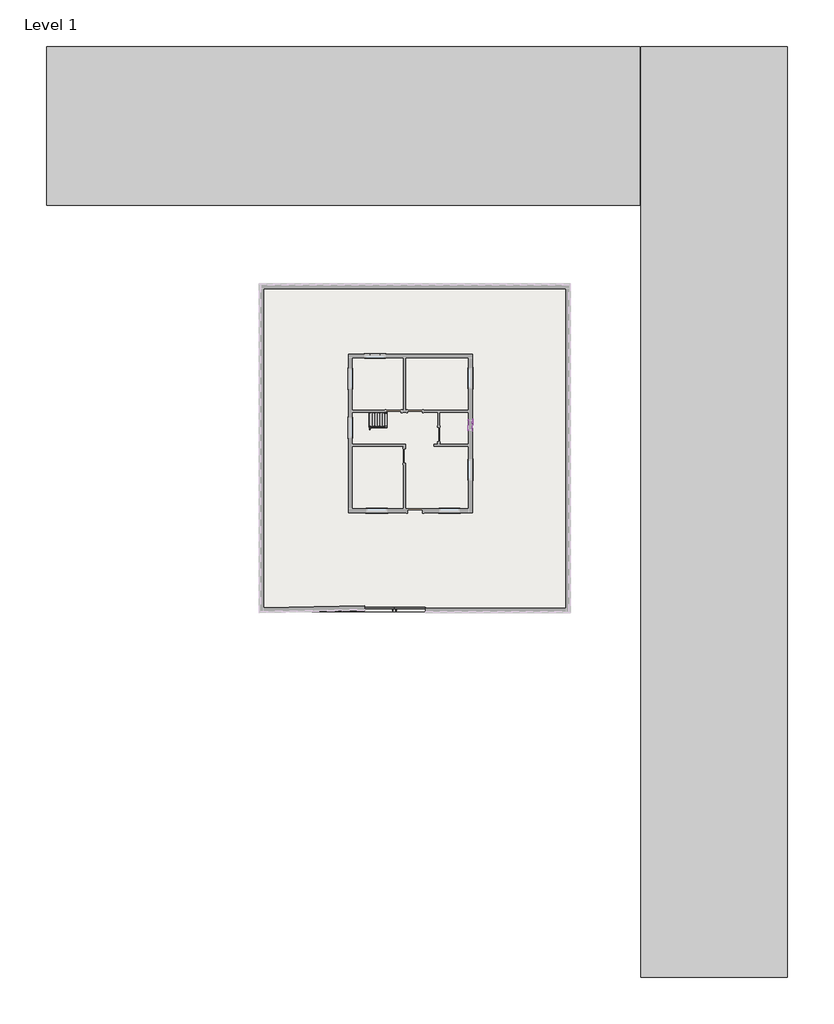
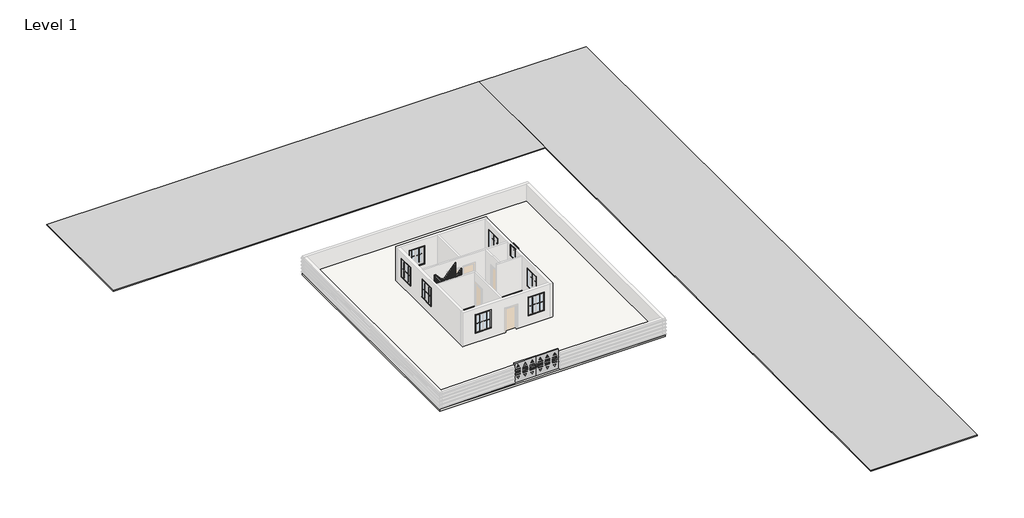
# One storey, part 2 of 2: 35 proxies, 3 members, 2 railings, 1 slab, 1 stair flight.
"""IFC4 building model written with IfcOpenShell, lengths in millimetres."""

from ifc_helpers import new_model, si_unit, frame, origin, place, context, project, spatial, polyline, outline, extrude, faceted_brep, transform, mapped, element, save
from components import generic_models_afecbd1f, generic_models_1_generic_models_1_344866f9, generic_models_2_generic_models_2_ab047e66, muntin_pattern_2x2_muntin_pattern_2x2_6dad3731, muntin_pattern_2x2_muntin_pattern_2x2_a30a3345, muntin_pattern_2x2_muntin_pattern_2x2_53152e2c, muntin_pattern_2x2_muntin_pattern_2x2_e8f3e573, trim_window_exterior_flat_with_sill_92b9b949, trim_window_exterior_flat_with_sill_a665a915, trim_window_interior_flat_picture_frame_3bb882cf, trim_window_interior_flat_picture_frame_d485c387, stair_flight_41b76c56

model = new_model("IFC4")

# Units and contexts
model_context = context("Model", 3, world=origin())
ifc_project = project(units=[si_unit("LENGTHUNIT", "METRE", prefix="MILLI")], contexts=[model_context])

# Site, building, storey
site = spatial("IfcSite", under=ifc_project)
building = spatial("IfcBuilding", under=site)
storey = spatial("IfcBuildingStorey", under=building, Name="Level 1", Elevation=0.0)

# Proxies
placement = place(None, origin())
generic_models_shape = generic_models_afecbd1f(model_context)
element("IfcBuildingElementProxy", 1, Name="Generic Models", at=placement, inside=storey, context=model_context, shape_type="MappedRepresentation", body=[
    mapped(generic_models_shape, transform((3790.95, -1079.5, 0.0), x_axis=(1.0, 0.0, 0.0), y_axis=(0.0, 1.0, 0.0), z_axis=(0.0, 0.0, 1.0))),
])
generic_models_1_generic_models_1_shape = generic_models_1_generic_models_1_344866f9(model_context)
element("IfcBuildingElementProxy", 2, Name="Generic Models 1 : Generic Models 1", ObjectType="Generic Models 1 : Generic Models 1", at=placement, inside=storey, context=model_context, shape_type="MappedRepresentation", body=[
    mapped(generic_models_1_generic_models_1_shape, transform((0.0, 0.0, 0.0), x_axis=(1.0, 0.0, 0.0), y_axis=(0.0, 1.0, 0.0), z_axis=(0.0, 0.0, 1.0))),
])
generic_models_2_generic_models_2_shape = generic_models_2_generic_models_2_ab047e66(model_context)
element("IfcBuildingElementProxy", 3, Name="Generic Models 2 : Generic Models 2", ObjectType="Generic Models 2 : Generic Models 2", at=placement, inside=storey, context=model_context, shape_type="MappedRepresentation", body=[
    mapped(generic_models_2_generic_models_2_shape, transform((0.0, 0.0, 0.0), x_axis=(1.0, 0.0, 0.0), y_axis=(0.0, 1.0, 0.0), z_axis=(0.0, 0.0, 1.0))),
])
muntin_pattern_2x2_muntin_pattern_2x2_shape = muntin_pattern_2x2_muntin_pattern_2x2_6dad3731(model_context)
element("IfcBuildingElementProxy", 4, Name="Muntin Pattern_2x2 : Muntin Pattern_2x2", ObjectType="Muntin Pattern_2x2 : Muntin Pattern_2x2", at=placement, inside=storey, context=model_context, shape_type="MappedRepresentation", body=[
    mapped(muntin_pattern_2x2_muntin_pattern_2x2_shape, transform((2601.9125, 14468.475, 984.25), x_axis=(1.0, 0.0, 0.0), y_axis=(0.0, 1.0, 0.0), z_axis=(0.0, 0.0, 1.0))),
])
element("IfcBuildingElementProxy", 5, Name="Muntin Pattern_2x2 : Muntin Pattern_2x2", ObjectType="Muntin Pattern_2x2 : Muntin Pattern_2x2", at=placement, inside=storey, context=model_context, shape_type="MappedRepresentation", body=[
    mapped(muntin_pattern_2x2_muntin_pattern_2x2_shape, transform((8880.475, 13295.3125, 984.25), x_axis=(0.0, -1.0, 0.0), y_axis=(1.0, 0.0, 0.0), z_axis=(0.0, 0.0, 1.0))),
])
element("IfcBuildingElementProxy", 6, Name="Muntin Pattern_2x2 : Muntin Pattern_2x2", ObjectType="Muntin Pattern_2x2 : Muntin Pattern_2x2", at=placement, inside=storey, context=model_context, shape_type="MappedRepresentation", body=[
    mapped(muntin_pattern_2x2_muntin_pattern_2x2_shape, transform((8880.475, 7662.8625, 984.25), x_axis=(0.0, -1.0, 0.0), y_axis=(1.0, 0.0, 0.0), z_axis=(0.0, 0.0, 1.0))),
])
element("IfcBuildingElementProxy", 7, Name="Muntin Pattern_2x2 : Muntin Pattern_2x2", ObjectType="Muntin Pattern_2x2 : Muntin Pattern_2x2", at=placement, inside=storey, context=model_context, shape_type="MappedRepresentation", body=[
    mapped(muntin_pattern_2x2_muntin_pattern_2x2_shape, transform((7785.1, 4733.925, 984.25), x_axis=(-1.0, 0.0, 0.0), y_axis=(0.0, -1.0, 0.0), z_axis=(0.0, 0.0, 1.0))),
])
element("IfcBuildingElementProxy", 8, Name="Muntin Pattern_2x2 : Muntin Pattern_2x2", ObjectType="Muntin Pattern_2x2 : Muntin Pattern_2x2", at=placement, inside=storey, context=model_context, shape_type="MappedRepresentation", body=[
    mapped(muntin_pattern_2x2_muntin_pattern_2x2_shape, transform((3313.1125, 4733.925, 984.25), x_axis=(-1.0, 0.0, 0.0), y_axis=(0.0, -1.0, 0.0), z_axis=(0.0, 0.0, 1.0))),
])
element("IfcBuildingElementProxy", 9, Name="Muntin Pattern_2x2 : Muntin Pattern_2x2", ObjectType="Muntin Pattern_2x2 : Muntin Pattern_2x2", at=placement, inside=storey, context=model_context, shape_type="MappedRepresentation", body=[
    mapped(muntin_pattern_2x2_muntin_pattern_2x2_shape, transform((1279.525, 9647.2375, 984.25), x_axis=(0.0, 1.0, 0.0), y_axis=(-1.0, 0.0, 0.0), z_axis=(0.0, 0.0, 1.0))),
])
element("IfcBuildingElementProxy", 10, Name="Muntin Pattern_2x2 : Muntin Pattern_2x2", ObjectType="Muntin Pattern_2x2 : Muntin Pattern_2x2", at=placement, inside=storey, context=model_context, shape_type="MappedRepresentation", body=[
    mapped(muntin_pattern_2x2_muntin_pattern_2x2_shape, transform((1279.525, 12657.1375, 984.25), x_axis=(0.0, 1.0, 0.0), y_axis=(-1.0, 0.0, 0.0), z_axis=(0.0, 0.0, 1.0))),
])
muntin_pattern_2x2_muntin_pattern_2x2_2_shape = muntin_pattern_2x2_muntin_pattern_2x2_a30a3345(model_context)
element("IfcBuildingElementProxy", 11, Name="Muntin Pattern_2x2 : Muntin Pattern_2x2", ObjectType="Muntin Pattern_2x2 : Muntin Pattern_2x2", at=placement, inside=storey, context=model_context, shape_type="MappedRepresentation", body=[
    mapped(muntin_pattern_2x2_muntin_pattern_2x2_2_shape, transform((3208.3375, 14468.475, 984.25), x_axis=(-1.0, 0.0, 0.0), y_axis=(0.0, -1.0, 0.0), z_axis=(0.0, 0.0, 1.0))),
])
element("IfcBuildingElementProxy", 12, Name="Muntin Pattern_2x2 : Muntin Pattern_2x2", ObjectType="Muntin Pattern_2x2 : Muntin Pattern_2x2", at=placement, inside=storey, context=model_context, shape_type="MappedRepresentation", body=[
    mapped(muntin_pattern_2x2_muntin_pattern_2x2_2_shape, transform((8880.475, 12688.8875, 984.25), x_axis=(0.0, 1.0, 0.0), y_axis=(-1.0, 0.0, 0.0), z_axis=(0.0, 0.0, 1.0))),
])
element("IfcBuildingElementProxy", 13, Name="Muntin Pattern_2x2 : Muntin Pattern_2x2", ObjectType="Muntin Pattern_2x2 : Muntin Pattern_2x2", at=placement, inside=storey, context=model_context, shape_type="MappedRepresentation", body=[
    mapped(muntin_pattern_2x2_muntin_pattern_2x2_2_shape, transform((8880.475, 7056.4375, 984.25), x_axis=(0.0, 1.0, 0.0), y_axis=(-1.0, 0.0, 0.0), z_axis=(0.0, 0.0, 1.0))),
])
element("IfcBuildingElementProxy", 14, Name="Muntin Pattern_2x2 : Muntin Pattern_2x2", ObjectType="Muntin Pattern_2x2 : Muntin Pattern_2x2", at=placement, inside=storey, context=model_context, shape_type="MappedRepresentation", body=[
    mapped(muntin_pattern_2x2_muntin_pattern_2x2_2_shape, transform((7178.675, 4733.925, 984.25), x_axis=(1.0, 0.0, 0.0), y_axis=(0.0, 1.0, 0.0), z_axis=(0.0, 0.0, 1.0))),
])
element("IfcBuildingElementProxy", 15, Name="Muntin Pattern_2x2 : Muntin Pattern_2x2", ObjectType="Muntin Pattern_2x2 : Muntin Pattern_2x2", at=placement, inside=storey, context=model_context, shape_type="MappedRepresentation", body=[
    mapped(muntin_pattern_2x2_muntin_pattern_2x2_2_shape, transform((2706.6875, 4733.925, 984.25), x_axis=(1.0, 0.0, 0.0), y_axis=(0.0, 1.0, 0.0), z_axis=(0.0, 0.0, 1.0))),
])
element("IfcBuildingElementProxy", 16, Name="Muntin Pattern_2x2 : Muntin Pattern_2x2", ObjectType="Muntin Pattern_2x2 : Muntin Pattern_2x2", at=placement, inside=storey, context=model_context, shape_type="MappedRepresentation", body=[
    mapped(muntin_pattern_2x2_muntin_pattern_2x2_2_shape, transform((1279.525, 10253.6625, 984.25), x_axis=(0.0, -1.0, 0.0), y_axis=(1.0, 0.0, 0.0), z_axis=(0.0, 0.0, 1.0))),
])
element("IfcBuildingElementProxy", 17, Name="Muntin Pattern_2x2 : Muntin Pattern_2x2", ObjectType="Muntin Pattern_2x2 : Muntin Pattern_2x2", at=placement, inside=storey, context=model_context, shape_type="MappedRepresentation", body=[
    mapped(muntin_pattern_2x2_muntin_pattern_2x2_2_shape, transform((1279.525, 13263.5625, 984.25), x_axis=(0.0, -1.0, 0.0), y_axis=(1.0, 0.0, 0.0), z_axis=(0.0, 0.0, 1.0))),
])
muntin_pattern_2x2_muntin_pattern_2x2_3_shape = muntin_pattern_2x2_muntin_pattern_2x2_53152e2c(model_context)
element("IfcBuildingElementProxy", 18, Name="Muntin Pattern_2x2 : Muntin Pattern_2x2", ObjectType="Muntin Pattern_2x2 : Muntin Pattern_2x2", at=placement, inside=storey, context=model_context, shape_type="MappedRepresentation", body=[
    mapped(muntin_pattern_2x2_muntin_pattern_2x2_3_shape, transform((8880.475, 10266.3625, 2203.45), x_axis=(0.0, -1.0, 0.0), y_axis=(1.0, 0.0, 0.0), z_axis=(0.0, 0.0, 1.0))),
])
muntin_pattern_2x2_muntin_pattern_2x2_4_shape = muntin_pattern_2x2_muntin_pattern_2x2_e8f3e573(model_context)
element("IfcBuildingElementProxy", 19, Name="Muntin Pattern_2x2 : Muntin Pattern_2x2", ObjectType="Muntin Pattern_2x2 : Muntin Pattern_2x2", at=placement, inside=storey, context=model_context, shape_type="MappedRepresentation", body=[
    mapped(muntin_pattern_2x2_muntin_pattern_2x2_4_shape, transform((8880.475, 9964.7375, 2203.45), x_axis=(0.0, 1.0, 0.0), y_axis=(-1.0, 0.0, 0.0), z_axis=(0.0, 0.0, 1.0))),
])
trim_window_exterior_flat_with_sill_shape = trim_window_exterior_flat_with_sill_92b9b949(model_context)
element("IfcBuildingElementProxy", 20, Name="Trim-Window-Exterior-Flat : with Sill", ObjectType="Trim-Window-Exterior-Flat : with Sill", at=placement, inside=storey, context=model_context, shape_type="MappedRepresentation", body=[
    mapped(trim_window_exterior_flat_with_sill_shape, transform((2905.125, 14478.0, 2438.4), x_axis=(-1.0, 0.0, 0.0), y_axis=(0.0, 0.0, 1.0), z_axis=(0.0, 1.0, 0.0))),
])
element("IfcBuildingElementProxy", 21, Name="Trim-Window-Exterior-Flat : with Sill", ObjectType="Trim-Window-Exterior-Flat : with Sill", at=placement, inside=storey, context=model_context, shape_type="MappedRepresentation", body=[
    mapped(trim_window_exterior_flat_with_sill_shape, transform((8890.0, 12992.1, 2438.4), x_axis=(0.0, 1.0, 0.0), y_axis=(0.0, 0.0, 1.0), z_axis=(1.0, 0.0, 0.0))),
])
element("IfcBuildingElementProxy", 22, Name="Trim-Window-Exterior-Flat : with Sill", ObjectType="Trim-Window-Exterior-Flat : with Sill", at=placement, inside=storey, context=model_context, shape_type="MappedRepresentation", body=[
    mapped(trim_window_exterior_flat_with_sill_shape, transform((8890.0, 7359.65, 2438.4), x_axis=(0.0, 1.0, 0.0), y_axis=(0.0, 0.0, 1.0), z_axis=(1.0, 0.0, 0.0))),
])
element("IfcBuildingElementProxy", 23, Name="Trim-Window-Exterior-Flat : with Sill", ObjectType="Trim-Window-Exterior-Flat : with Sill", at=placement, inside=storey, context=model_context, shape_type="MappedRepresentation", body=[
    mapped(trim_window_exterior_flat_with_sill_shape, transform((7481.8875, 4724.4, 2438.4), x_axis=(1.0, 0.0, 0.0), y_axis=(0.0, 0.0, 1.0), z_axis=(0.0, -1.0, 0.0))),
])
element("IfcBuildingElementProxy", 24, Name="Trim-Window-Exterior-Flat : with Sill", ObjectType="Trim-Window-Exterior-Flat : with Sill", at=placement, inside=storey, context=model_context, shape_type="MappedRepresentation", body=[
    mapped(trim_window_exterior_flat_with_sill_shape, transform((3009.9, 4724.4, 2438.4), x_axis=(1.0, 0.0, 0.0), y_axis=(0.0, 0.0, 1.0), z_axis=(0.0, -1.0, 0.0))),
])
element("IfcBuildingElementProxy", 25, Name="Trim-Window-Exterior-Flat : with Sill", ObjectType="Trim-Window-Exterior-Flat : with Sill", at=placement, inside=storey, context=model_context, shape_type="MappedRepresentation", body=[
    mapped(trim_window_exterior_flat_with_sill_shape, transform((1270.0, 9950.45, 2438.4), x_axis=(0.0, -1.0, 0.0), y_axis=(0.0, 0.0, 1.0), z_axis=(-1.0, 0.0, 0.0))),
])
element("IfcBuildingElementProxy", 26, Name="Trim-Window-Exterior-Flat : with Sill", ObjectType="Trim-Window-Exterior-Flat : with Sill", at=placement, inside=storey, context=model_context, shape_type="MappedRepresentation", body=[
    mapped(trim_window_exterior_flat_with_sill_shape, transform((1270.0, 12960.35, 2438.4), x_axis=(0.0, -1.0, 0.0), y_axis=(0.0, 0.0, 1.0), z_axis=(-1.0, 0.0, 0.0))),
])
trim_window_exterior_flat_with_sill_2_shape = trim_window_exterior_flat_with_sill_a665a915(model_context)
element("IfcBuildingElementProxy", 27, Name="Trim-Window-Exterior-Flat : with Sill", ObjectType="Trim-Window-Exterior-Flat : with Sill", at=placement, inside=storey, context=model_context, shape_type="MappedRepresentation", body=[
    mapped(trim_window_exterior_flat_with_sill_2_shape, transform((8890.0, 10115.55, 3048.0), x_axis=(0.0, 1.0, 0.0), y_axis=(0.0, 0.0, 1.0), z_axis=(1.0, 0.0, 0.0))),
])
trim_window_interior_flat_picture_frame_shape = trim_window_interior_flat_picture_frame_3bb882cf(model_context)
element("IfcBuildingElementProxy", 28, Name="Trim-Window-Interior-Flat : Picture Frame", ObjectType="Trim-Window-Interior-Flat : Picture Frame", at=placement, inside=storey, context=model_context, shape_type="MappedRepresentation", body=[
    mapped(trim_window_interior_flat_picture_frame_shape, transform((2905.125, 14249.4, 2438.4), x_axis=(1.0, 0.0, 0.0), y_axis=(0.0, 0.0, 1.0), z_axis=(0.0, -1.0, 0.0))),
])
element("IfcBuildingElementProxy", 29, Name="Trim-Window-Interior-Flat : Picture Frame", ObjectType="Trim-Window-Interior-Flat : Picture Frame", at=placement, inside=storey, context=model_context, shape_type="MappedRepresentation", body=[
    mapped(trim_window_interior_flat_picture_frame_shape, transform((8661.4, 12992.1, 2438.4), x_axis=(0.0, -1.0, 0.0), y_axis=(0.0, 0.0, 1.0), z_axis=(-1.0, 0.0, 0.0))),
])
element("IfcBuildingElementProxy", 30, Name="Trim-Window-Interior-Flat : Picture Frame", ObjectType="Trim-Window-Interior-Flat : Picture Frame", at=placement, inside=storey, context=model_context, shape_type="MappedRepresentation", body=[
    mapped(trim_window_interior_flat_picture_frame_shape, transform((8661.4, 7359.65, 2438.4), x_axis=(0.0, -1.0, 0.0), y_axis=(0.0, 0.0, 1.0), z_axis=(-1.0, 0.0, 0.0))),
])
element("IfcBuildingElementProxy", 31, Name="Trim-Window-Interior-Flat : Picture Frame", ObjectType="Trim-Window-Interior-Flat : Picture Frame", at=placement, inside=storey, context=model_context, shape_type="MappedRepresentation", body=[
    mapped(trim_window_interior_flat_picture_frame_shape, transform((7481.8875, 4953.0, 2438.4), x_axis=(-1.0, 0.0, 0.0), y_axis=(0.0, 0.0, 1.0), z_axis=(0.0, 1.0, 0.0))),
])
element("IfcBuildingElementProxy", 32, Name="Trim-Window-Interior-Flat : Picture Frame", ObjectType="Trim-Window-Interior-Flat : Picture Frame", at=placement, inside=storey, context=model_context, shape_type="MappedRepresentation", body=[
    mapped(trim_window_interior_flat_picture_frame_shape, transform((3009.9, 4953.0, 2438.4), x_axis=(-1.0, 0.0, 0.0), y_axis=(0.0, 0.0, 1.0), z_axis=(0.0, 1.0, 0.0))),
])
element("IfcBuildingElementProxy", 33, Name="Trim-Window-Interior-Flat : Picture Frame", ObjectType="Trim-Window-Interior-Flat : Picture Frame", at=placement, inside=storey, context=model_context, shape_type="MappedRepresentation", body=[
    mapped(trim_window_interior_flat_picture_frame_shape, transform((1498.6, 9950.45, 2438.4), x_axis=(0.0, 1.0, 0.0), y_axis=(0.0, 0.0, 1.0), z_axis=(1.0, 0.0, 0.0))),
])
element("IfcBuildingElementProxy", 34, Name="Trim-Window-Interior-Flat : Picture Frame", ObjectType="Trim-Window-Interior-Flat : Picture Frame", at=placement, inside=storey, context=model_context, shape_type="MappedRepresentation", body=[
    mapped(trim_window_interior_flat_picture_frame_shape, transform((1498.6, 12960.35, 2438.4), x_axis=(0.0, 1.0, 0.0), y_axis=(0.0, 0.0, 1.0), z_axis=(1.0, 0.0, 0.0))),
])
trim_window_interior_flat_picture_frame_2_shape = trim_window_interior_flat_picture_frame_d485c387(model_context)
element("IfcBuildingElementProxy", 35, Name="Trim-Window-Interior-Flat : Picture Frame", ObjectType="Trim-Window-Interior-Flat : Picture Frame", at=placement, inside=storey, context=model_context, shape_type="MappedRepresentation", body=[
    mapped(trim_window_interior_flat_picture_frame_2_shape, transform((8661.4, 10115.55, 3048.0), x_axis=(0.0, -1.0, 0.0), y_axis=(0.0, 0.0, 1.0), z_axis=(-1.0, 0.0, 0.0))),
])

# Members
element("IfcMember", 36, ObjectType="Stringer - 2\" Width", at=placement, inside=storey, context=model_context, shape_type="SweptSolid", body=[
    extrude(outline(polyline([(0.0, 3632.2), (274.6288314, 3632.2), (1403.5177203, 2616.2), (947.8883192, 2616.2), (0.0, 3469.2994873), (0.0, 3632.2)])), frame((0.0, 9944.1, 0.0), z_axis=(0.0, 1.0, 0.0), x_axis=(0.0, 0.0, 1.0)), (0.0, 0.0, 1.0), 50.8),
])
element("IfcMember", 37, ObjectType="Stringer - 2\" Width", at=placement, inside=storey, context=model_context, shape_type="SweptSolid", body=[
    extrude(outline(polyline([(2565.4, 9994.9), (2616.2, 9994.9), (2616.2, 9893.3), (2565.4, 9893.3), (2565.4, 9994.9)])), frame((0.0, 0.0, 1126.0666667), z_axis=(0.0, 0.0, 1.0), x_axis=(1.0, 0.0, 0.0)), (0.0, 0.0, 1.0), 304.8),
])
element("IfcMember", 38, ObjectType="Stringer - 2\" Width", at=placement, inside=storey, context=model_context, shape_type="SweptSolid", body=[
    extrude(outline(polyline([(1629.2954981, 2565.4), (1173.666097, 2565.4), (2358.9994303, 3632.2), (2814.6288314, 3632.2), (1629.2954981, 2565.4)])), frame((0.0, 9842.5, 0.0), z_axis=(0.0, 1.0, 0.0), x_axis=(0.0, 0.0, 1.0)), (0.0, 0.0, 1.0), 50.8),
])

# Railings
element("IfcRailing", 39, ObjectType="Handrail - Rectangular", at=placement, inside=storey, context=model_context, shape_type="SolidModel", body=[
    faceted_brep([(3632.2, 10858.5, 1083.7333333), (3632.2, 10858.5, 1007.7950998), (3632.2, 10909.3, 1007.7950998), (3632.2, 10909.3, 1083.7333333), (2565.4, 10858.5, 2269.0666667), (2542.7755898, 10858.5, 2218.2666667), (2542.7755898, 10909.3, 2218.2666667), (2565.4, 10909.3, 2269.0666667), (2463.8, 10858.5, 2269.0666667), (2463.8, 10858.5, 2218.2666667), (2413.0, 10909.3, 2218.2666667), (2413.0, 10909.3, 2269.0666667), (2463.8, 9055.1, 2269.0666667), (2463.8, 9004.3, 2218.2666667), (2413.0, 9004.3, 2218.2666667), (2413.0, 9055.1, 2269.0666667), (2463.8, 9055.1, 2410.1777778), (2463.8, 9004.3, 2359.3777778), (2413.0, 9004.3, 2359.3777778), (2413.0, 9055.1, 2410.1777778), (2463.8, 8978.9, 2410.1777778), (2463.8, 8978.9, 2359.3777778), (2413.0, 8928.1, 2359.3777778), (2413.0, 8928.1, 2410.1777778), (2540.0, 8978.9, 2410.1777778), (2562.6244102, 8978.9, 2359.3777778), (2562.6244102, 8928.1, 2359.3777778), (2540.0, 8928.1, 2410.1777778), (3632.2, 8978.9, 3623.7333333), (3632.2, 8928.1, 3623.7333333), (3632.2, 8928.1, 3547.7950998), (3632.2, 8978.9, 3547.7950998)], [[[0, 1, 2, 3]], [[1, 0, 4, 5]], [[2, 1, 5, 6]], [[3, 2, 6, 7]], [[0, 3, 7, 4]], [[5, 4, 8, 9]], [[6, 5, 9, 10]], [[7, 6, 10, 11]], [[4, 7, 11, 8]], [[9, 8, 12, 13]], [[10, 9, 13, 14]], [[11, 10, 14, 15]], [[8, 11, 15, 12]], [[13, 12, 16, 17]], [[14, 13, 17, 18]], [[15, 14, 18, 19]], [[12, 15, 19, 16]], [[17, 16, 20, 21]], [[18, 17, 21, 22]], [[19, 18, 22, 23]], [[16, 19, 23, 20]], [[21, 20, 24, 25]], [[22, 21, 25, 26]], [[23, 22, 26, 27]], [[20, 23, 27, 24]], [[28, 29, 30, 31]], [[25, 24, 28, 31]], [[26, 25, 31, 30]], [[27, 26, 30, 29]], [[24, 27, 29, 28]]]),
    extrude(outline(polyline([(3473.7117665, 3565.525), (3452.5450998, 3546.475), (2540.0, 3546.475), (2540.0, 3565.525), (3473.7117665, 3565.525)])), frame((0.0, 8943.975, 0.0), z_axis=(0.0, 1.0, 0.0), x_axis=(0.0, 0.0, 1.0)), (0.0, 0.0, 1.0), 19.05),
    extrude(outline(polyline([(3360.8228776, 3463.925), (3339.6562109, 3444.875), (2370.6666667, 3444.875), (2370.6666667, 3463.925), (3360.8228776, 3463.925)])), frame((0.0, 8943.975, 0.0), z_axis=(0.0, 1.0, 0.0), x_axis=(0.0, 0.0, 1.0)), (0.0, 0.0, 1.0), 19.05),
    extrude(outline(polyline([(3247.9339887, 3362.325), (3226.767322, 3343.275), (2370.6666667, 3343.275), (2370.6666667, 3362.325), (3247.9339887, 3362.325)])), frame((0.0, 8943.975, 0.0), z_axis=(0.0, 1.0, 0.0), x_axis=(0.0, 0.0, 1.0)), (0.0, 0.0, 1.0), 19.05),
    extrude(outline(polyline([(3135.0450998, 3260.725), (3113.8784332, 3241.675), (2201.3333333, 3241.675), (2201.3333333, 3260.725), (3135.0450998, 3260.725)])), frame((0.0, 8943.975, 0.0), z_axis=(0.0, 1.0, 0.0), x_axis=(0.0, 0.0, 1.0)), (0.0, 0.0, 1.0), 19.05),
    extrude(outline(polyline([(3022.1562109, 3159.125), (3000.9895443, 3140.075), (2032.0, 3140.075), (2032.0, 3159.125), (3022.1562109, 3159.125)])), frame((0.0, 8943.975, 0.0), z_axis=(0.0, 1.0, 0.0), x_axis=(0.0, 0.0, 1.0)), (0.0, 0.0, 1.0), 19.05),
    extrude(outline(polyline([(2909.267322, 3057.525), (2888.1006554, 3038.475), (2032.0, 3038.475), (2032.0, 3057.525), (2909.267322, 3057.525)])), frame((0.0, 8943.975, 0.0), z_axis=(0.0, 1.0, 0.0), x_axis=(0.0, 0.0, 1.0)), (0.0, 0.0, 1.0), 19.05),
    extrude(outline(polyline([(2796.3784332, 2955.925), (2775.2117665, 2936.875), (1862.6666667, 2936.875), (1862.6666667, 2955.925), (2796.3784332, 2955.925)])), frame((0.0, 8943.975, 0.0), z_axis=(0.0, 1.0, 0.0), x_axis=(0.0, 0.0, 1.0)), (0.0, 0.0, 1.0), 19.05),
    extrude(outline(polyline([(2683.4895443, 2854.325), (2662.3228776, 2835.275), (1693.3333333, 2835.275), (1693.3333333, 2854.325), (2683.4895443, 2854.325)])), frame((0.0, 8943.975, 0.0), z_axis=(0.0, 1.0, 0.0), x_axis=(0.0, 0.0, 1.0)), (0.0, 0.0, 1.0), 19.05),
    extrude(outline(polyline([(2570.6006554, 2752.725), (2549.4339887, 2733.675), (1693.3333333, 2733.675), (1693.3333333, 2752.725), (2570.6006554, 2752.725)])), frame((0.0, 8943.975, 0.0), z_axis=(0.0, 1.0, 0.0), x_axis=(0.0, 0.0, 1.0)), (0.0, 0.0, 1.0), 19.05),
    extrude(outline(polyline([(2457.7117665, 2651.125), (2436.5450998, 2632.075), (1524.0, 2632.075), (1524.0, 2651.125), (2457.7117665, 2651.125)])), frame((0.0, 8943.975, 0.0), z_axis=(0.0, 1.0, 0.0), x_axis=(0.0, 0.0, 1.0)), (0.0, 0.0, 1.0), 19.05),
    extrude(outline(polyline([(2344.8228776, 2549.525), (2323.6562109, 2530.475), (1354.6666667, 2530.475), (1354.6666667, 2549.525), (2344.8228776, 2549.525)])), frame((0.0, 8943.975, 0.0), z_axis=(0.0, 1.0, 0.0), x_axis=(0.0, 0.0, 1.0)), (0.0, 0.0, 1.0), 19.05),
    extrude(outline(polyline([(2428.875, 9064.625), (2447.925, 9064.625), (2447.925, 9045.575), (2428.875, 9045.575), (2428.875, 9064.625)])), frame((0.0, 0.0, 1354.6666667), z_axis=(0.0, 0.0, 1.0), x_axis=(1.0, 0.0, 0.0)), (0.0, 0.0, 1.0), 863.6),
    extrude(outline(polyline([(2428.875, 9166.225), (2447.925, 9166.225), (2447.925, 9147.175), (2428.875, 9147.175), (2428.875, 9166.225)])), frame((0.0, 0.0, 1354.6666667), z_axis=(0.0, 0.0, 1.0), x_axis=(1.0, 0.0, 0.0)), (0.0, 0.0, 1.0), 863.6),
    extrude(outline(polyline([(2428.875, 9267.825), (2447.925, 9267.825), (2447.925, 9248.775), (2428.875, 9248.775), (2428.875, 9267.825)])), frame((0.0, 0.0, 1354.6666667), z_axis=(0.0, 0.0, 1.0), x_axis=(1.0, 0.0, 0.0)), (0.0, 0.0, 1.0), 863.6),
    extrude(outline(polyline([(2428.875, 9369.425), (2447.925, 9369.425), (2447.925, 9350.375), (2428.875, 9350.375), (2428.875, 9369.425)])), frame((0.0, 0.0, 1354.6666667), z_axis=(0.0, 0.0, 1.0), x_axis=(1.0, 0.0, 0.0)), (0.0, 0.0, 1.0), 863.6),
    extrude(outline(polyline([(2428.875, 9471.025), (2447.925, 9471.025), (2447.925, 9451.975), (2428.875, 9451.975), (2428.875, 9471.025)])), frame((0.0, 0.0, 1354.6666667), z_axis=(0.0, 0.0, 1.0), x_axis=(1.0, 0.0, 0.0)), (0.0, 0.0, 1.0), 863.6),
    extrude(outline(polyline([(2428.875, 9572.625), (2447.925, 9572.625), (2447.925, 9553.575), (2428.875, 9553.575), (2428.875, 9572.625)])), frame((0.0, 0.0, 1354.6666667), z_axis=(0.0, 0.0, 1.0), x_axis=(1.0, 0.0, 0.0)), (0.0, 0.0, 1.0), 863.6),
    extrude(outline(polyline([(2428.875, 9674.225), (2447.925, 9674.225), (2447.925, 9655.175), (2428.875, 9655.175), (2428.875, 9674.225)])), frame((0.0, 0.0, 1354.6666667), z_axis=(0.0, 0.0, 1.0), x_axis=(1.0, 0.0, 0.0)), (0.0, 0.0, 1.0), 863.6),
    extrude(outline(polyline([(2428.875, 9775.825), (2447.925, 9775.825), (2447.925, 9756.775), (2428.875, 9756.775), (2428.875, 9775.825)])), frame((0.0, 0.0, 1354.6666667), z_axis=(0.0, 0.0, 1.0), x_axis=(1.0, 0.0, 0.0)), (0.0, 0.0, 1.0), 863.6),
    extrude(outline(polyline([(2428.875, 9877.425), (2447.925, 9877.425), (2447.925, 9858.375), (2428.875, 9858.375), (2428.875, 9877.425)])), frame((0.0, 0.0, 1354.6666667), z_axis=(0.0, 0.0, 1.0), x_axis=(1.0, 0.0, 0.0)), (0.0, 0.0, 1.0), 863.6),
    extrude(outline(polyline([(2428.875, 9979.025), (2447.925, 9979.025), (2447.925, 9959.975), (2428.875, 9959.975), (2428.875, 9979.025)])), frame((0.0, 0.0, 1354.6666667), z_axis=(0.0, 0.0, 1.0), x_axis=(1.0, 0.0, 0.0)), (0.0, 0.0, 1.0), 863.6),
    extrude(outline(polyline([(2428.875, 10080.625), (2447.925, 10080.625), (2447.925, 10061.575), (2428.875, 10061.575), (2428.875, 10080.625)])), frame((0.0, 0.0, 1354.6666667), z_axis=(0.0, 0.0, 1.0), x_axis=(1.0, 0.0, 0.0)), (0.0, 0.0, 1.0), 863.6),
    extrude(outline(polyline([(2428.875, 10182.225), (2447.925, 10182.225), (2447.925, 10163.175), (2428.875, 10163.175), (2428.875, 10182.225)])), frame((0.0, 0.0, 1354.6666667), z_axis=(0.0, 0.0, 1.0), x_axis=(1.0, 0.0, 0.0)), (0.0, 0.0, 1.0), 863.6),
    extrude(outline(polyline([(2428.875, 10283.825), (2447.925, 10283.825), (2447.925, 10264.775), (2428.875, 10264.775), (2428.875, 10283.825)])), frame((0.0, 0.0, 1354.6666667), z_axis=(0.0, 0.0, 1.0), x_axis=(1.0, 0.0, 0.0)), (0.0, 0.0, 1.0), 863.6),
    extrude(outline(polyline([(2428.875, 10385.425), (2447.925, 10385.425), (2447.925, 10366.375), (2428.875, 10366.375), (2428.875, 10385.425)])), frame((0.0, 0.0, 1354.6666667), z_axis=(0.0, 0.0, 1.0), x_axis=(1.0, 0.0, 0.0)), (0.0, 0.0, 1.0), 863.6),
    extrude(outline(polyline([(2428.875, 10487.025), (2447.925, 10487.025), (2447.925, 10467.975), (2428.875, 10467.975), (2428.875, 10487.025)])), frame((0.0, 0.0, 1354.6666667), z_axis=(0.0, 0.0, 1.0), x_axis=(1.0, 0.0, 0.0)), (0.0, 0.0, 1.0), 863.6),
    extrude(outline(polyline([(2428.875, 10588.625), (2447.925, 10588.625), (2447.925, 10569.575), (2428.875, 10569.575), (2428.875, 10588.625)])), frame((0.0, 0.0, 1354.6666667), z_axis=(0.0, 0.0, 1.0), x_axis=(1.0, 0.0, 0.0)), (0.0, 0.0, 1.0), 863.6),
    extrude(outline(polyline([(2428.875, 10690.225), (2447.925, 10690.225), (2447.925, 10671.175), (2428.875, 10671.175), (2428.875, 10690.225)])), frame((0.0, 0.0, 1354.6666667), z_axis=(0.0, 0.0, 1.0), x_axis=(1.0, 0.0, 0.0)), (0.0, 0.0, 1.0), 863.6),
    extrude(outline(polyline([(2428.875, 10791.825), (2447.925, 10791.825), (2447.925, 10772.775), (2428.875, 10772.775), (2428.875, 10791.825)])), frame((0.0, 0.0, 1354.6666667), z_axis=(0.0, 0.0, 1.0), x_axis=(1.0, 0.0, 0.0)), (0.0, 0.0, 1.0), 863.6),
    extrude(outline(polyline([(2524.125, 10893.425), (2524.125, 10874.375), (2505.075, 10874.375), (2505.075, 10893.425), (2524.125, 10893.425)])), frame((0.0, 0.0, 1354.6666667), z_axis=(0.0, 0.0, 1.0), x_axis=(1.0, 0.0, 0.0)), (0.0, 0.0, 1.0), 863.6),
    extrude(outline(polyline([(2126.1006554, 2625.725), (2147.267322, 2606.675), (1185.3333333, 2606.675), (1185.3333333, 2625.725), (2126.1006554, 2625.725)])), frame((0.0, 10874.375, 0.0), z_axis=(0.0, 1.0, 0.0), x_axis=(0.0, 0.0, 1.0)), (0.0, 0.0, 1.0), 19.05),
    extrude(outline(polyline([(2013.2117665, 2727.325), (2034.3784332, 2708.275), (1185.3333333, 2708.275), (1185.3333333, 2727.325), (2013.2117665, 2727.325)])), frame((0.0, 10874.375, 0.0), z_axis=(0.0, 1.0, 0.0), x_axis=(0.0, 0.0, 1.0)), (0.0, 0.0, 1.0), 19.05),
    extrude(outline(polyline([(1900.3228776, 2828.925), (1921.4895443, 2809.875), (1016.0, 2809.875), (1016.0, 2828.925), (1900.3228776, 2828.925)])), frame((0.0, 10874.375, 0.0), z_axis=(0.0, 1.0, 0.0), x_axis=(0.0, 0.0, 1.0)), (0.0, 0.0, 1.0), 19.05),
    extrude(outline(polyline([(1787.4339887, 2930.525), (1808.6006554, 2911.475), (846.6666667, 2911.475), (846.6666667, 2930.525), (1787.4339887, 2930.525)])), frame((0.0, 10874.375, 0.0), z_axis=(0.0, 1.0, 0.0), x_axis=(0.0, 0.0, 1.0)), (0.0, 0.0, 1.0), 19.05),
    extrude(outline(polyline([(1674.5450998, 3032.125), (1695.7117665, 3013.075), (846.6666667, 3013.075), (846.6666667, 3032.125), (1674.5450998, 3032.125)])), frame((0.0, 10874.375, 0.0), z_axis=(0.0, 1.0, 0.0), x_axis=(0.0, 0.0, 1.0)), (0.0, 0.0, 1.0), 19.05),
    extrude(outline(polyline([(1561.6562109, 3133.725), (1582.8228776, 3114.675), (677.3333333, 3114.675), (677.3333333, 3133.725), (1561.6562109, 3133.725)])), frame((0.0, 10874.375, 0.0), z_axis=(0.0, 1.0, 0.0), x_axis=(0.0, 0.0, 1.0)), (0.0, 0.0, 1.0), 19.05),
    extrude(outline(polyline([(1448.767322, 3235.325), (1469.9339887, 3216.275), (508.0, 3216.275), (508.0, 3235.325), (1448.767322, 3235.325)])), frame((0.0, 10874.375, 0.0), z_axis=(0.0, 1.0, 0.0), x_axis=(0.0, 0.0, 1.0)), (0.0, 0.0, 1.0), 19.05),
    extrude(outline(polyline([(1335.8784332, 3336.925), (1357.0450998, 3317.875), (508.0, 3317.875), (508.0, 3336.925), (1335.8784332, 3336.925)])), frame((0.0, 10874.375, 0.0), z_axis=(0.0, 1.0, 0.0), x_axis=(0.0, 0.0, 1.0)), (0.0, 0.0, 1.0), 19.05),
    extrude(outline(polyline([(1222.9895443, 3438.525), (1244.1562109, 3419.475), (338.6666667, 3419.475), (338.6666667, 3438.525), (1222.9895443, 3438.525)])), frame((0.0, 10874.375, 0.0), z_axis=(0.0, 1.0, 0.0), x_axis=(0.0, 0.0, 1.0)), (0.0, 0.0, 1.0), 19.05),
    extrude(outline(polyline([(1110.1006554, 3540.125), (1131.267322, 3521.075), (169.3333333, 3521.075), (169.3333333, 3540.125), (1110.1006554, 3540.125)])), frame((0.0, 10874.375, 0.0), z_axis=(0.0, 1.0, 0.0), x_axis=(0.0, 0.0, 1.0)), (0.0, 0.0, 1.0), 19.05),
    extrude(outline(polyline([(2428.875, 8963.025), (2447.925, 8963.025), (2447.925, 8943.975), (2428.875, 8943.975), (2428.875, 8963.025)])), frame((0.0, 0.0, 1354.6666667), z_axis=(0.0, 0.0, 1.0), x_axis=(1.0, 0.0, 0.0)), (0.0, 0.0, 1.0), 1004.7111111),
    extrude(outline(polyline([(2447.925, 10893.425), (2447.925, 10874.375), (2428.875, 10874.375), (2428.875, 10893.425), (2447.925, 10893.425)])), frame((0.0, 0.0, 1354.6666667), z_axis=(0.0, 0.0, 1.0), x_axis=(1.0, 0.0, 0.0)), (0.0, 0.0, 1.0), 863.6),
    extrude(outline(polyline([(3547.7950998, 3632.2), (3526.6284332, 3613.15), (2540.0, 3613.15), (2540.0, 3632.2), (3547.7950998, 3632.2)])), frame((0.0, 8943.975, 0.0), z_axis=(0.0, 1.0, 0.0), x_axis=(0.0, 0.0, 1.0)), (0.0, 0.0, 1.0), 19.05),
    extrude(outline(polyline([(1007.7950998, 3632.2), (1028.9617665, 3613.15), (169.3333333, 3613.15), (169.3333333, 3632.2), (1007.7950998, 3632.2)])), frame((0.0, 10874.375, 0.0), z_axis=(0.0, 1.0, 0.0), x_axis=(0.0, 0.0, 1.0)), (0.0, 0.0, 1.0), 19.05),
])
element("IfcRailing", 40, ObjectType="Handrail - Rectangular", at=placement, inside=storey, context=model_context, shape_type="SolidModel", body=[
    faceted_brep([(3632.2, 9994.9, 1083.7333333), (3632.2, 9994.9, 1007.7950998), (3632.2, 10045.7, 1007.7950998), (3632.2, 10045.7, 1083.7333333), (2641.6, 9994.9, 2184.4), (2590.8, 9994.9, 2164.9062109), (2590.8, 10045.7, 2164.9062109), (2641.6, 10045.7, 2184.4), (2641.6, 9994.9, 2269.0666667), (2590.8, 9994.9, 2218.2666667), (2590.8, 10045.7, 2218.2666667), (2641.6, 10045.7, 2269.0666667), (2565.4, 9994.9, 2269.0666667), (2565.4, 9994.9, 2218.2666667), (2514.6, 10045.7, 2218.2666667), (2514.6, 10045.7, 2269.0666667), (2565.4, 9918.7, 2269.0666667), (2565.4, 9867.9, 2218.2666667), (2514.6, 9867.9, 2218.2666667), (2514.6, 9918.7, 2269.0666667), (2565.4, 9918.7, 2523.0666667), (2565.4, 9867.9, 2472.2666667), (2514.6, 9867.9, 2472.2666667), (2514.6, 9918.7, 2523.0666667), (2565.4, 9842.5, 2523.0666667), (2565.4, 9842.5, 2472.2666667), (2514.6, 9791.7, 2472.2666667), (2514.6, 9791.7, 2523.0666667), (2641.6, 9842.5, 2523.0666667), (2664.2244102, 9842.5, 2472.2666667), (2664.2244102, 9791.7, 2472.2666667), (2641.6, 9791.7, 2523.0666667), (3632.2, 9842.5, 3623.7333333), (3632.2, 9791.7, 3623.7333333), (3632.2, 9791.7, 3547.7950998), (3632.2, 9842.5, 3547.7950998)], [[[0, 1, 2, 3]], [[1, 0, 4, 5]], [[2, 1, 5, 6]], [[3, 2, 6, 7]], [[0, 3, 7, 4]], [[5, 4, 8, 9]], [[6, 5, 9, 10]], [[7, 6, 10, 11]], [[4, 7, 11, 8]], [[9, 8, 12, 13]], [[10, 9, 13, 14]], [[11, 10, 14, 15]], [[8, 11, 15, 12]], [[13, 12, 16, 17]], [[14, 13, 17, 18]], [[15, 14, 18, 19]], [[12, 15, 19, 16]], [[17, 16, 20, 21]], [[18, 17, 21, 22]], [[19, 18, 22, 23]], [[16, 19, 23, 20]], [[21, 20, 24, 25]], [[22, 21, 25, 26]], [[23, 22, 26, 27]], [[20, 23, 27, 24]], [[25, 24, 28, 29]], [[26, 25, 29, 30]], [[27, 26, 30, 31]], [[24, 27, 31, 28]], [[32, 33, 34, 35]], [[29, 28, 32, 35]], [[30, 29, 35, 34]], [[31, 30, 34, 33]], [[28, 31, 33, 32]]]),
    extrude(outline(polyline([(3452.5450998, 3546.475), (2540.0, 3546.475), (2540.0, 3565.525), (3473.7117665, 3565.525), (3452.5450998, 3546.475)])), frame((0.0, 9807.575, 0.0), z_axis=(0.0, 1.0, 0.0), x_axis=(0.0, 0.0, 1.0)), (0.0, 0.0, 1.0), 19.05),
    extrude(outline(polyline([(3339.6562109, 3444.875), (2370.6666667, 3444.875), (2370.6666667, 3463.925), (3360.8228776, 3463.925), (3339.6562109, 3444.875)])), frame((0.0, 9807.575, 0.0), z_axis=(0.0, 1.0, 0.0), x_axis=(0.0, 0.0, 1.0)), (0.0, 0.0, 1.0), 19.05),
    extrude(outline(polyline([(3226.767322, 3343.275), (2370.6666667, 3343.275), (2370.6666667, 3362.325), (3247.9339887, 3362.325), (3226.767322, 3343.275)])), frame((0.0, 9807.575, 0.0), z_axis=(0.0, 1.0, 0.0), x_axis=(0.0, 0.0, 1.0)), (0.0, 0.0, 1.0), 19.05),
    extrude(outline(polyline([(3113.8784332, 3241.675), (2201.3333333, 3241.675), (2201.3333333, 3260.725), (3135.0450998, 3260.725), (3113.8784332, 3241.675)])), frame((0.0, 9807.575, 0.0), z_axis=(0.0, 1.0, 0.0), x_axis=(0.0, 0.0, 1.0)), (0.0, 0.0, 1.0), 19.05),
    extrude(outline(polyline([(3000.9895443, 3140.075), (2032.0, 3140.075), (2032.0, 3159.125), (3022.1562109, 3159.125), (3000.9895443, 3140.075)])), frame((0.0, 9807.575, 0.0), z_axis=(0.0, 1.0, 0.0), x_axis=(0.0, 0.0, 1.0)), (0.0, 0.0, 1.0), 19.05),
    extrude(outline(polyline([(2888.1006554, 3038.475), (2032.0, 3038.475), (2032.0, 3057.525), (2909.267322, 3057.525), (2888.1006554, 3038.475)])), frame((0.0, 9807.575, 0.0), z_axis=(0.0, 1.0, 0.0), x_axis=(0.0, 0.0, 1.0)), (0.0, 0.0, 1.0), 19.05),
    extrude(outline(polyline([(2775.2117665, 2936.875), (1862.6666667, 2936.875), (1862.6666667, 2955.925), (2796.3784332, 2955.925), (2775.2117665, 2936.875)])), frame((0.0, 9807.575, 0.0), z_axis=(0.0, 1.0, 0.0), x_axis=(0.0, 0.0, 1.0)), (0.0, 0.0, 1.0), 19.05),
    extrude(outline(polyline([(2662.3228776, 2835.275), (1693.3333333, 2835.275), (1693.3333333, 2854.325), (2683.4895443, 2854.325), (2662.3228776, 2835.275)])), frame((0.0, 9807.575, 0.0), z_axis=(0.0, 1.0, 0.0), x_axis=(0.0, 0.0, 1.0)), (0.0, 0.0, 1.0), 19.05),
    extrude(outline(polyline([(2549.4339887, 2733.675), (1693.3333333, 2733.675), (1693.3333333, 2752.725), (2570.6006554, 2752.725), (2549.4339887, 2733.675)])), frame((0.0, 9807.575, 0.0), z_axis=(0.0, 1.0, 0.0), x_axis=(0.0, 0.0, 1.0)), (0.0, 0.0, 1.0), 19.05),
    extrude(outline(polyline([(2436.5450998, 2632.075), (1524.0, 2632.075), (1524.0, 2651.125), (2457.7117665, 2651.125), (2436.5450998, 2632.075)])), frame((0.0, 9807.575, 0.0), z_axis=(0.0, 1.0, 0.0), x_axis=(0.0, 0.0, 1.0)), (0.0, 0.0, 1.0), 19.05),
    extrude(outline(polyline([(2549.525, 9928.225), (2549.525, 9909.175), (2530.475, 9909.175), (2530.475, 9928.225), (2549.525, 9928.225)])), frame((0.0, 0.0, 1354.6666667), z_axis=(0.0, 0.0, 1.0), x_axis=(1.0, 0.0, 0.0)), (0.0, 0.0, 1.0), 863.6),
    extrude(outline(polyline([(2625.725, 10010.775), (2606.675, 10010.775), (2606.675, 10029.825), (2625.725, 10029.825), (2625.725, 10010.775)])), frame((0.0, 0.0, 1185.3333333), z_axis=(0.0, 0.0, 1.0), x_axis=(1.0, 0.0, 0.0)), (0.0, 0.0, 1.0), 1032.9333333),
    extrude(outline(polyline([(2034.3784332, 2708.275), (1185.3333333, 2708.275), (1185.3333333, 2727.325), (2013.2117665, 2727.325), (2034.3784332, 2708.275)])), frame((0.0, 10010.775, 0.0), z_axis=(0.0, 1.0, 0.0), x_axis=(0.0, 0.0, 1.0)), (0.0, 0.0, 1.0), 19.05),
    extrude(outline(polyline([(1921.4895443, 2809.875), (1016.0, 2809.875), (1016.0, 2828.925), (1900.3228776, 2828.925), (1921.4895443, 2809.875)])), frame((0.0, 10010.775, 0.0), z_axis=(0.0, 1.0, 0.0), x_axis=(0.0, 0.0, 1.0)), (0.0, 0.0, 1.0), 19.05),
    extrude(outline(polyline([(1808.6006554, 2911.475), (846.6666667, 2911.475), (846.6666667, 2930.525), (1787.4339887, 2930.525), (1808.6006554, 2911.475)])), frame((0.0, 10010.775, 0.0), z_axis=(0.0, 1.0, 0.0), x_axis=(0.0, 0.0, 1.0)), (0.0, 0.0, 1.0), 19.05),
    extrude(outline(polyline([(1695.7117665, 3013.075), (846.6666667, 3013.075), (846.6666667, 3032.125), (1674.5450998, 3032.125), (1695.7117665, 3013.075)])), frame((0.0, 10010.775, 0.0), z_axis=(0.0, 1.0, 0.0), x_axis=(0.0, 0.0, 1.0)), (0.0, 0.0, 1.0), 19.05),
    extrude(outline(polyline([(1582.8228776, 3114.675), (677.3333333, 3114.675), (677.3333333, 3133.725), (1561.6562109, 3133.725), (1582.8228776, 3114.675)])), frame((0.0, 10010.775, 0.0), z_axis=(0.0, 1.0, 0.0), x_axis=(0.0, 0.0, 1.0)), (0.0, 0.0, 1.0), 19.05),
    extrude(outline(polyline([(1469.9339887, 3216.275), (508.0, 3216.275), (508.0, 3235.325), (1448.767322, 3235.325), (1469.9339887, 3216.275)])), frame((0.0, 10010.775, 0.0), z_axis=(0.0, 1.0, 0.0), x_axis=(0.0, 0.0, 1.0)), (0.0, 0.0, 1.0), 19.05),
    extrude(outline(polyline([(1357.0450998, 3317.875), (508.0, 3317.875), (508.0, 3336.925), (1335.8784332, 3336.925), (1357.0450998, 3317.875)])), frame((0.0, 10010.775, 0.0), z_axis=(0.0, 1.0, 0.0), x_axis=(0.0, 0.0, 1.0)), (0.0, 0.0, 1.0), 19.05),
    extrude(outline(polyline([(1244.1562109, 3419.475), (338.6666667, 3419.475), (338.6666667, 3438.525), (1222.9895443, 3438.525), (1244.1562109, 3419.475)])), frame((0.0, 10010.775, 0.0), z_axis=(0.0, 1.0, 0.0), x_axis=(0.0, 0.0, 1.0)), (0.0, 0.0, 1.0), 19.05),
    extrude(outline(polyline([(1131.267322, 3521.075), (169.3333333, 3521.075), (169.3333333, 3540.125), (1110.1006554, 3540.125), (1131.267322, 3521.075)])), frame((0.0, 10010.775, 0.0), z_axis=(0.0, 1.0, 0.0), x_axis=(0.0, 0.0, 1.0)), (0.0, 0.0, 1.0), 19.05),
    extrude(outline(polyline([(2549.525, 9826.625), (2549.525, 9807.575), (2530.475, 9807.575), (2530.475, 9826.625), (2549.525, 9826.625)])), frame((0.0, 0.0, 1354.6666667), z_axis=(0.0, 0.0, 1.0), x_axis=(1.0, 0.0, 0.0)), (0.0, 0.0, 1.0), 1117.6),
    extrude(outline(polyline([(2549.525, 10010.775), (2530.475, 10010.775), (2530.475, 10029.825), (2549.525, 10029.825), (2549.525, 10010.775)])), frame((0.0, 0.0, 1354.6666667), z_axis=(0.0, 0.0, 1.0), x_axis=(1.0, 0.0, 0.0)), (0.0, 0.0, 1.0), 863.6),
    extrude(outline(polyline([(3526.6284332, 3613.15), (2540.0, 3613.15), (2540.0, 3632.2), (3547.7950998, 3632.2), (3526.6284332, 3613.15)])), frame((0.0, 9807.575, 0.0), z_axis=(0.0, 1.0, 0.0), x_axis=(0.0, 0.0, 1.0)), (0.0, 0.0, 1.0), 19.05),
    extrude(outline(polyline([(1028.9617665, 3613.15), (169.3333333, 3613.15), (169.3333333, 3632.2), (1007.7950998, 3632.2), (1028.9617665, 3613.15)])), frame((0.0, 10010.775, 0.0), z_axis=(0.0, 1.0, 0.0), x_axis=(0.0, 0.0, 1.0)), (0.0, 0.0, 1.0), 19.05),
])

# Slab
element("IfcSlab", 41, ObjectType="Generic - 12\"", at=placement, inside=storey, context=model_context, shape_type="SweptSolid", body=[
    extrude(outline(polyline([(14867.9342856, 18740.5705427), (14867.9342856, -1376.2294573), (-4182.0657144, -1376.2294573), (-4182.0657144, 18740.5705427), (14867.9342856, 18740.5705427)])), frame((0.0, 0.0, -152.4), z_axis=(0.0, 0.0, 1.0), x_axis=(1.0, 0.0, 0.0)), (0.0, 0.0, 1.0), 152.4),
])

# Stair flight
stair_flight_shape = stair_flight_41b76c56(model_context)
element("IfcStairFlight", 42, ObjectType="2\" Tread 1\" Nosing 1/4\" Riser", at=placement, inside=storey, context=model_context, shape_type="MappedRepresentation", body=[
    mapped(stair_flight_shape, transform((0.0, 0.0, 0.0), x_axis=(1.0, 0.0, 0.0), y_axis=(0.0, 1.0, 0.0), z_axis=(0.0, 0.0, 1.0))),
])

save(model, "model.ifc")

# Revit data of these elements
# Type
#   Default Elevation = 0
# Type "Muntin Pattern_2x2 : Muntin Pattern_2x2"
#   Width [instance default] = 4' - 0"
#   Thickness = 0' - 0 1/2"
#   Height [instance default] = 4' - 0"
#   Distance = 0' - 0 3/4"
#   Interior Material [instance default] = none
#   Exterior Material [instance default] = none
#   Default Elevation = 0
# Type "Trim-Window-Exterior-Flat : with Sill"
#   Trim Width = 0' - 2 1/4"
#   Trim Thickness_Picture Frame = 0' - 1 1/4"
#   Trim Thickness_with Sill = 0' - 0 3/4"
#   Sill Thickness = 0' - 1 1/4"
#   Opening Width [instance default] = 2' - 0"
#   Opening Height [instance default] = 3' - 0"
#   Default Elevation = 4' - 0"
#   Sill = yes
#   Picture Frame = no
#   Trim Material [instance default] = none
# Type "Trim-Window-Interior-Flat : Picture Frame"
#   Trim Thickness_Picture Frame = 0' - 1 1/4"
#   Trim Width = 0' - 2 1/4"
#   Trim Thickness_with Sill = 0' - 0 3/4"
#   Sill Thickness = 0' - 1 1/4"
#   Opening Width [instance default] = 2' - 0"
#   Opening Height [instance default] = 3' - 0"
#   Default Elevation = 4' - 0"
#   Sill = no
#   Picture Frame = yes
#   Trim Material [instance default] = none
# Type "Handrail - Rectangular"
#   Assembly Code = "C2010400"
#   built-in parameter 1008612 = 0.0416667 (stored number, unit not read)
#   built-in parameter 1008611 = 0.0416667 (stored number, unit not read)
#   built-in parameter 1008609 = 0.333333 (stored number, unit not read)
#   built-in parameter 1008604 = 0.166667 (stored number, unit not read)
#   built-in parameter 1008603 = 0.166667 (stored number, unit not read)
#   Railing Height = 3' - 0"
#   built-in parameter 1008630 = 2
#   built-in parameter 1008610 = 2
#   built-in parameter 1008618 = Baluster - Square : 3/4"
# Type "Generic - 12\""
#   Assembly Code = "B1010"
#   Function = 0
#   Layers, outside or top first: 0' - 6" no material (function 1)
# Element 1 (IfcBuildingElementProxy)
#   Phase Created = New Construction
#   Materials on its faces: "GATE"
# Element 2 (IfcBuildingElementProxy, "Generic Models 1 : Generic Models 1")
#   Phase Created = New Construction
# Element 3 (IfcBuildingElementProxy, "Generic Models 2 : Generic Models 2")
#   Phase Created = New Construction
# Elements 4, 5, 6, 7, 8, 9, 10, 11, 12, 13, 14, 15, 16, 17 (IfcBuildingElementProxy, "Muntin Pattern_2x2 : Muntin Pattern_2x2")
#   Width = 1' - 6 5/8"
#   Height = 4' - 6 1/2"
#   Interior Material = Wood - Stained
#   Exterior Material = Clad - White
#   Phase Created = New Construction
#   Materials on its faces: "Clad - White", "Wood - Stained"
# Elements 18, 19 (IfcBuildingElementProxy, "Muntin Pattern_2x2 : Muntin Pattern_2x2")
#   Width = 0' - 6 5/8"
#   Height = 2' - 6 1/2"
#   Interior Material = Wood - Stained
#   Exterior Material = Clad - White
#   Phase Created = New Construction
#   Materials on its faces: "Clad - White", "Wood - Stained"
# Elements 20, 21, 22, 23, 24, 25, 26 (IfcBuildingElementProxy, "Trim-Window-Exterior-Flat : with Sill")
#   Opening Width = 4' - 0"
#   Opening Height = 5' - 0"
#   Trim Material = Clad - White
#   Phase Created = New Construction
#   Materials on its faces: "Clad - White"
# Element 27 (IfcBuildingElementProxy, "Trim-Window-Exterior-Flat : with Sill")
#   Opening Width = 2' - 0"
#   Opening Height = 3' - 0"
#   Trim Material = Clad - White
#   Phase Created = New Construction
#   Materials on its faces: "Clad - White"
# Elements 28, 29, 30, 31, 32, 33, 34 (IfcBuildingElementProxy, "Trim-Window-Interior-Flat : Picture Frame")
#   Opening Width = 4' - 0"
#   Opening Height = 5' - 0"
#   Trim Material = Wood - Stained
#   Phase Created = New Construction
#   Materials on its faces: "Wood - Stained"
# Element 35 (IfcBuildingElementProxy, "Trim-Window-Interior-Flat : Picture Frame")
#   Opening Width = 2' - 0"
#   Opening Height = 3' - 0"
#   Trim Material = Wood - Stained
#   Phase Created = New Construction
#   Materials on its faces: "Wood - Stained"
# Elements 36, 37, 38 (IfcMember, "Stringer - 2\" Width")
#   Phase Created = New Construction
# Elements 39, 40 (IfcRailing, "Handrail - Rectangular")
#   Phase Created = New Construction
# Element 41 (IfcSlab, "Generic - 12\"")
#   Height Offset From Level = 0' - 0"
#   Phase Created = New Construction
#   Materials on its faces: "Textile - Linen, Smooth", "Default Floor", "Wood - Stained"
# Element 42 (IfcStairFlight, "2\" Tread 1\" Nosing 1/4\" Riser")
#   Phase Created = New Construction
# Materials
#   "GATE": class "Generic", colour RGB 120 120 120, transparency 0, Cost = 0
#   "Clad - White": class "Wood", colour RGB 242 242 238, transparency 0, Cost = 0
#   "Wood - Stained": class "Wood", colour RGB 224 178 126, transparency 0, Cost = 0
#   "Textile - Linen, Smooth": colour RGB 249 239 230, transparency 0
#   "Default Floor": colour RGB 128 128 128, transparency 0, Cost = 0
